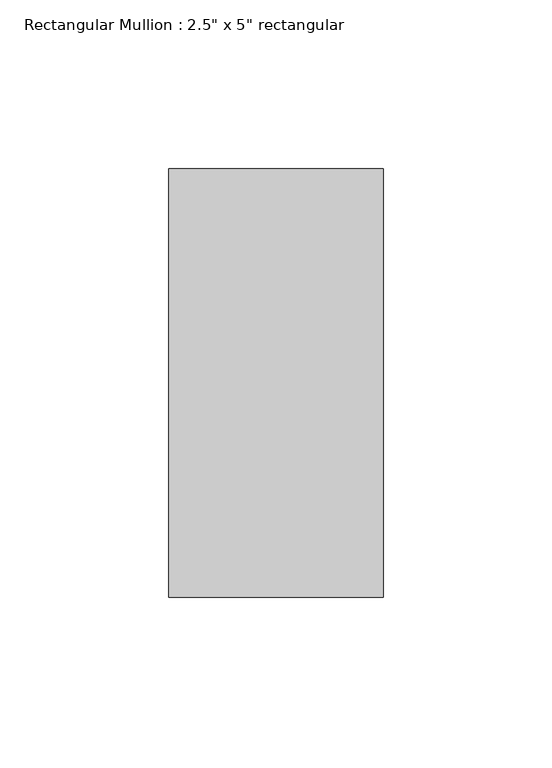
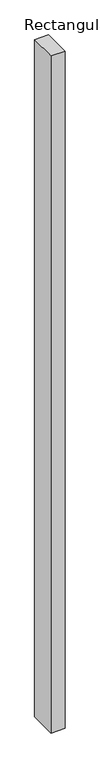
"""IFC4 building model written with IfcOpenShell, lengths in millimetres: member geometry."""

from ifc_helpers import new_model, si_unit, frame, origin, place, context, project, spatial, polyline, outline, extrude, source, transform, mapped, element, save


def member_3c8bcf7e(model_context):
    return source(origin(), model_context, "Body", "SweptSolid", [
        extrude(outline(polyline([(0.0, 63.5), (0.0, -63.5), (-63.5, -63.5), (-63.5, 63.5), (0.0, 63.5)])), frame((0.0, 0.0, -3232.15), z_axis=(0.0, 0.0, 1.0), x_axis=(1.0, 0.0, 0.0)), (0.0, 0.0, 1.0), 3232.15),
    ])


if __name__ == "__main__":
    model = new_model("IFC4")
    model_context = context("Model", 3, world=origin())
    ifc_project = project(units=[si_unit("LENGTHUNIT", "METRE", prefix="MILLI")], contexts=[model_context])
    site = spatial("IfcSite", under=ifc_project)
    building = spatial("IfcBuilding", under=site)
    placement = place(None, origin())
    member_shape = member_3c8bcf7e(model_context)
    element("IfcMember", 1, ObjectType="Rectangular Mullion : 2.5\" x 5\" rectangular", at=placement, inside=building, context=model_context, shape_type="MappedRepresentation", body=[
        mapped(member_shape, transform((0.0, 0.0, 0.0), x_axis=(1.0, 0.0, 0.0), y_axis=(0.0, 1.0, 0.0), z_axis=(0.0, 0.0, 1.0))),
    ])
    save(model, "model.ifc")

# Revit data of these elements
# Type "Rectangular Mullion : 2.5\" x 5\" rectangular"
#   built-in parameter 1007304 = 0.416667 (stored number, unit not read)
#   built-in parameter 1007301 = 0.104167 (stored number, unit not read)
#   built-in parameter 1007300 = 0.104167 (stored number, unit not read)
# Element 1 (IfcMember, "Rectangular Mullion : 2.5\" x 5\" rectangular")
#   Materials on its faces: "Iron, Ductile"
# Materials
#   "Iron, Ductile": class "Metal", colour RGB 0 0 0, transparency 0, Description = "Ductile cast iron", Cost = 0
